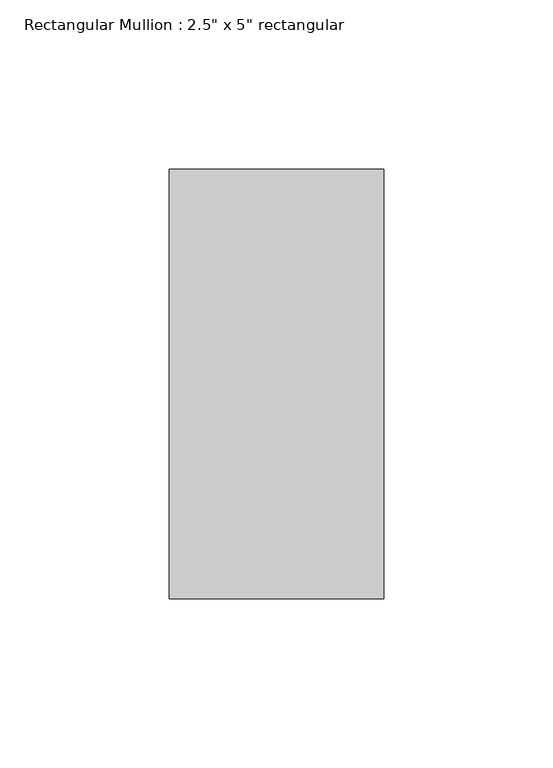
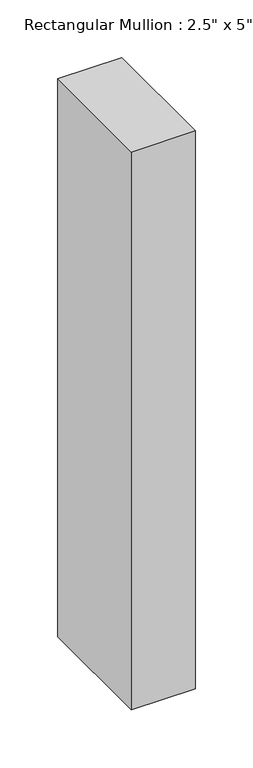
"""IFC4 building model written with IfcOpenShell, lengths in millimetres: member geometry."""

from ifc_helpers import new_model, si_unit, frame, origin, place, context, project, spatial, polyline, outline, extrude, source, transform, mapped, element, save


def member_9202991e(model_context):
    return source(origin(), model_context, "Body", "SweptSolid", [
        extrude(outline(polyline([(0.0, 63.5), (0.0, -63.5), (-63.5, -63.5), (-63.5, 63.5), (0.0, 63.5)])), frame((0.0, 0.0, -588.4333331), z_axis=(0.0, 0.0, 1.0), x_axis=(1.0, 0.0, 0.0)), (0.0, 0.0, 1.0), 588.4333331),
    ])


if __name__ == "__main__":
    model = new_model("IFC4")
    model_context = context("Model", 3, world=origin())
    ifc_project = project(units=[si_unit("LENGTHUNIT", "METRE", prefix="MILLI")], contexts=[model_context])
    site = spatial("IfcSite", under=ifc_project)
    building = spatial("IfcBuilding", under=site)
    placement = place(None, origin())
    member_shape = member_9202991e(model_context)
    element("IfcMember", 1, ObjectType="Rectangular Mullion : 2.5\" x 5\" rectangular", at=placement, inside=building, context=model_context, shape_type="MappedRepresentation", body=[
        mapped(member_shape, transform((0.0, 0.0, 0.0), x_axis=(1.0, 0.0, 0.0), y_axis=(0.0, 1.0, 0.0), z_axis=(0.0, 0.0, 1.0))),
    ])
    save(model, "model.ifc")

# Revit data of these elements
# Type "Rectangular Mullion : 2.5\" x 5\" rectangular"
#   built-in parameter 1007304 = 0.416667 (stored number, unit not read)
#   built-in parameter 1007301 = 0.104167 (stored number, unit not read)
#   built-in parameter 1007300 = 0.104167 (stored number, unit not read)
# Element 1 (IfcMember, "Rectangular Mullion : 2.5\" x 5\" rectangular")
#   Materials on its faces: "Aluminum"
# Materials
#   "Aluminum": class "Metal", colour RGB 247 247 247, transparency 0, Description = "Aluminum 6061", Cost = 0
